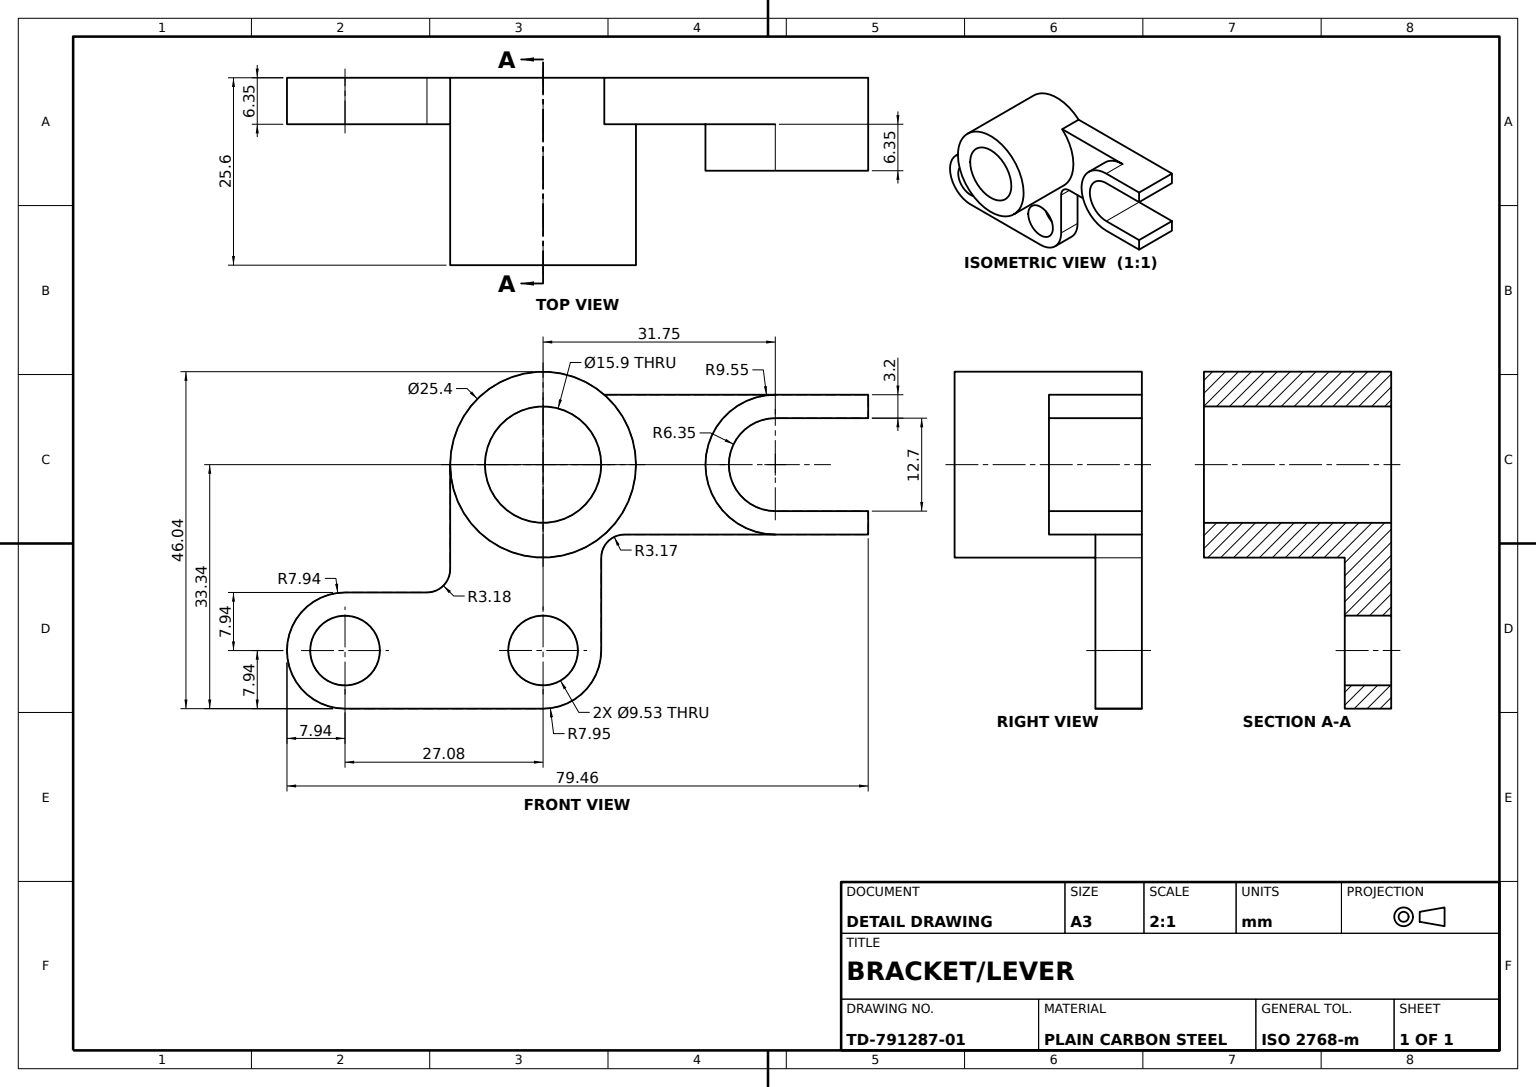
from build123d import *

# Parameters (mm, degrees)
HUB_TUBE_SKETCH_R   = 12.7
HUB_TUBE_SKETCH_R_2 = 7.9502
HUB_TUBE_DEPTH      = 25.6032
WEB_BOSS_DEPTH      = 12.7
FORK_EARS_SKETCH_R  = 4.7625
FORK_EARS_DEPTH     = 6.35


with BuildPart() as part:
    # Hub Tube Sketch → Hub Tube (new body)
    with BuildSketch(Plane.XY):
        Circle(HUB_TUBE_SKETCH_R)
        Circle(HUB_TUBE_SKETCH_R_2, mode=Mode.SUBTRACT)
    extrude(amount=HUB_TUBE_DEPTH)



with BuildPart() as body_2:
    # Web Boss Sketch → Web Boss (new body)
    with BuildSketch(Plane.XY):
        with BuildLine():
            Line((31.75, 9.5504), (44.45, 9.5504))
            Line((44.45, 9.5504), (44.45, 6.35))
            Line((44.45, 6.35), (31.75, 6.35))
            ThreePointArc((31.75, 6.35), (25.4, 0), (31.75, -6.35))
            Line((31.75, -6.35), (44.45, -6.35))
            Line((44.45, -6.35), (44.45, -9.5504))
            Line((44.45, -9.5504), (31.75, -9.5504))
            ThreePointArc((31.75, -9.5504), (22.1996, 0), (31.75, 9.5504))
        make_face()
    extrude(amount=WEB_BOSS_DEPTH)


with BuildPart() as part_1:
    add(part.part)

    add(body_2.part)  # Fork Ears merges body 2
    # Fork Ears Sketch → Fork Ears (add)
    with BuildSketch(Plane.XY):
        with BuildLine():
            Line((-12.7, 0), (-12.7, -14.2875))
            ThreePointArc((-12.7, -14.2875), (-13.62993597, -16.53256403), (-15.875, -17.4625))
            Line((-15.875, -17.4625), (-27.0764, -17.4625))
            ThreePointArc((-27.0764, -17.4625), (-35.0139, -25.4), (-27.0764, -33.3375))
            Line((-27.0764, -33.3375), (0, -33.3375))
            ThreePointArc((0, -33.3375), (5.621640332, -31.008940332), (7.9502, -25.3873))
            Line((7.9502, -25.3873), (7.9502, -12.7254))
            ThreePointArc((7.9502, -12.7254), (8.88013597, -10.48033597), (11.1252, -9.5504))
            Line((11.1252, -9.5504), (31.75, -9.5504))
            ThreePointArc((31.75, -9.5504), (22.1996, 0), (31.75, 9.5504))
            Line((31.75, 9.5504), (8.371371443, 9.5504))
            ThreePointArc((8.371371443, 9.5504), (5.242784693, -11.567333689), (-12.7, 0))
        make_face()
        with Locations((-27.0764, -25.4)):
            Circle(FORK_EARS_SKETCH_R, mode=Mode.SUBTRACT)
        with Locations((0, -25.3873)):
            Circle(FORK_EARS_SKETCH_R, mode=Mode.SUBTRACT)
    extrude(amount=FORK_EARS_DEPTH)


solid = part_1.part
